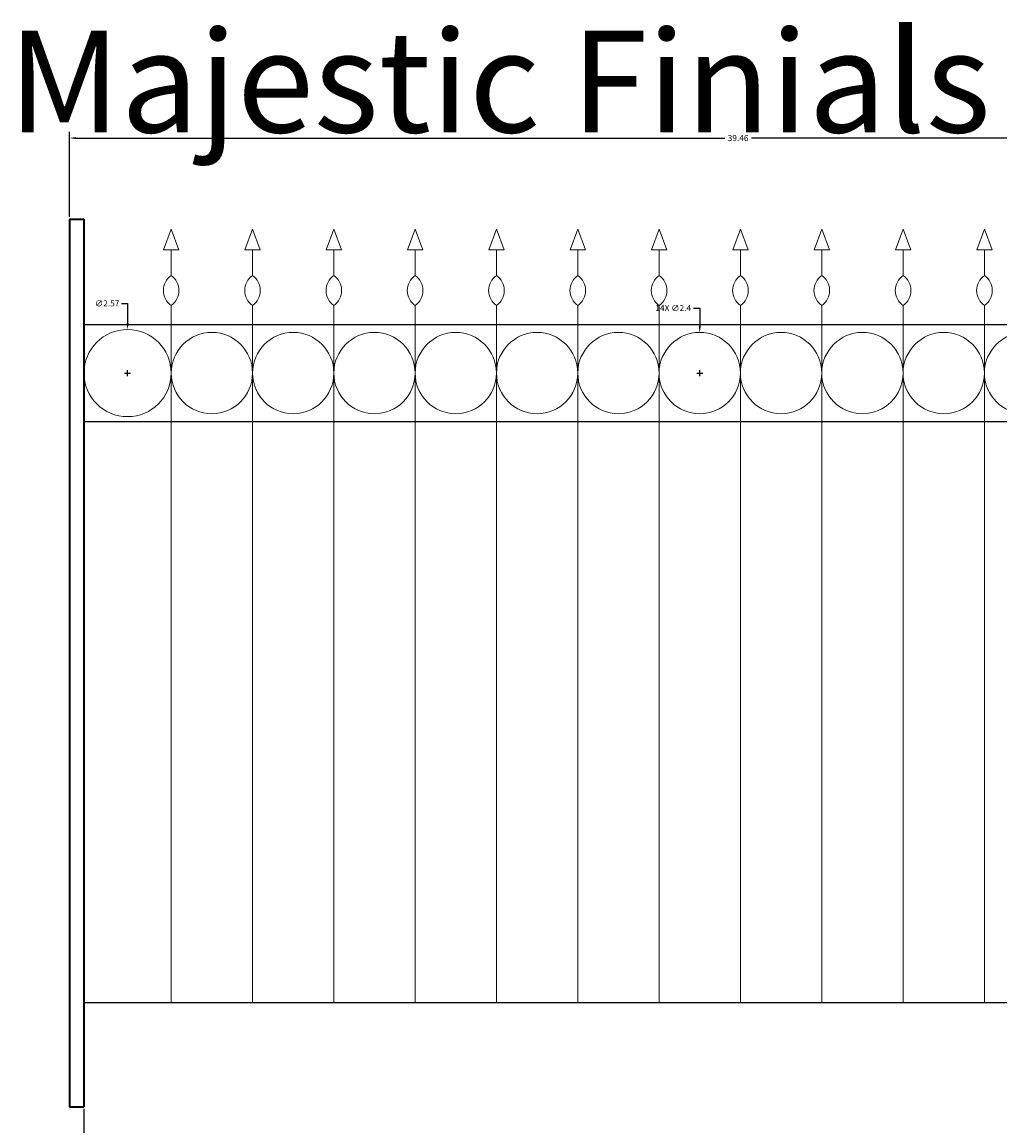
# Model space of a CAD drawing. Units: inches. Extents: x 756 to 915, y 488 to 695.
# Tile 5 of 25: x 815 to 844, y 512 to 545. Entities that reach past the tile are written whole.
import ezdxf

# ---------------------------------------------------------------- set-up
doc = ezdxf.new("R2010")
doc.units = ezdxf.units.IN
doc.header["$MEASUREMENT"] = 0
for name, color, linetype, lineweight in [('L-ANNO-TEXT', 7, 'Continuous', 25), ('L-FENC-PCKT', 7, 'Continuous', 18), ('L-FENC-POST', 7, 'Continuous', 35), ('L-FENC-RAIL', 7, 'Continuous', 25), ('L-FENC-RING', 7, 'Continuous', 18), ('M-DIMS', 2, 'Continuous', 18)]:
    doc.layers.add(name, color=color, linetype=linetype, lineweight=lineweight)
doc.styles.get("Standard").update_dxf_attribs({"font": 'arial.ttf'})
doc.dimstyles.get("Standard").update_dxf_attribs({"dimtxt": 0.18, "dimasz": 0.18, "dimexe": 0.18, "dimexo": 0.0625, "dimgap": 0.09, "dimtad": 0, "dimtih": 1, "dimtoh": 1, "dimdec": 0, "dimzin": 0, "dimdsep": 46, "dimlunit": 3, "dimtxsty": 'Standard', "dimcen": 0.09, "dimadec": 0, "dimazin": 0, "dimtfac": 1, "dimtdec": 0, "dimtofl": 0, "dimtmove": 0, "dimatfit": 3, "dimfxl": 1, "dimtolj": 1, "dimtzin": 0, "dimarcsym": 0})

# ---------------------------------------------------------------- blocks, each defined once
blk = doc.blocks.new('PICKET-MAJESTIC-FLUSH')
for p, q in [((0.231, 22.214), (0.231, 21.456)), ((0.231, 20.573), (0.231, 0))]:
    blk.add_line(p, q)
blk.add_lwpolyline([(0.231, 22.214), (0.004, 22.214), (0.231, 22.826), (0.458, 22.214)], close=True)
blk.add_lwpolyline([(0.231, 20.573, 0.522719), (0.231, 21.456, 0.522719)], format="xyb", close=True)
blk = doc.blocks.new('FENCE-POST-LEFT')
for p, q in [((0, 26.207), (0, 0)), ((0, 26.207), (0.426, 26.207)), ((0.426, 26.207), (0.426, 0)), ((0.426, 26.207), (0.426, 0)), ((0, 0), (0.426, 0))]:
    blk.add_line(p, q)
blk = doc.blocks.new('FENCE-PLUS-RING-BAND')
for centre, radius in [((1.286, 1.286), 1.286), ((3.773, 1.286), 1.2), ((6.173, 1.286), 1.2), ((8.572, 1.286), 1.2), ((10.972, 1.286), 1.2), ((13.372, 1.286), 1.2), ((15.772, 1.286), 1.2), ((18.172, 1.286), 1.2), ((20.572, 1.286), 1.2), ((22.972, 1.286), 1.2), ((25.372, 1.286), 1.2), ((27.772, 1.286), 1.2), ((30.172, 1.286), 1.2), ((32.572, 1.286), 1.2), ((34.971, 1.286), 1.2), ((37.388, 1.286), 1.217)]:
    blk.add_circle(centre, radius)
blk = doc.blocks.new('*D76')
at = {"layer": 'Defpoints', "color": 0, "transparency": 16777216}
for p in [(856.101, 541.142), (816.643, 538.752), (856.101, 538.752)]:
    blk.add_point(p, dxfattribs=at)
at = {"layer": 'M-DIMS', "color": 0, "lineweight": -2, "transparency": 16777216}
for p, q in [((816.643, 538.814), (816.643, 541.322)), ((856.101, 538.814), (856.101, 541.322)), ((816.823, 541.142), (835.978, 541.142)), ((855.921, 541.142), (836.765, 541.142))]:
    blk.add_line(p, q, dxfattribs=at)
at = {"layer": 'M-DIMS', "color": 0, "transparency": 16777216}
for points in [[(816.823, 541.172), (816.823, 541.112), (816.643, 541.142)], [(855.921, 541.172), (855.921, 541.112), (856.101, 541.142)]]:
    blk.add_solid(points, dxfattribs=at)
at = {"layer": 'M-DIMS', "color": 0, "transparency": 16777216, "insert": (836.372, 541.142), "char_height": 0.18, "attachment_point": 5}
blk.add_mtext('\\A1;39.46', dxfattribs=at)
blk = doc.blocks.new('*D78')
at = {"layer": 'Defpoints', "color": 0, "transparency": 16777216}
for p in [(817.069, 512.545), (855.674, 512.545), (855.674, 510.155)]:
    blk.add_point(p, dxfattribs=at)
at = {"layer": 'M-DIMS', "color": 0, "lineweight": -2, "transparency": 16777216}
for p, q in [((817.069, 512.482), (817.069, 509.975)), ((855.674, 512.482), (855.674, 509.975)), ((817.249, 510.155), (835.908, 510.155)), ((855.494, 510.155), (836.836, 510.155))]:
    blk.add_line(p, q, dxfattribs=at)
at = {"layer": 'M-DIMS', "color": 0, "transparency": 16777216}
for points in [[(817.249, 510.185), (817.249, 510.125), (817.069, 510.155)], [(855.494, 510.185), (855.494, 510.125), (855.674, 510.155)]]:
    blk.add_solid(points, dxfattribs=at)
at = {"layer": 'M-DIMS', "color": 0, "transparency": 16777216, "insert": (836.372, 510.155), "char_height": 0.18, "attachment_point": 5}
blk.add_mtext('\\A1;38.605', dxfattribs=at)
blk = doc.blocks.new('*D87')
at = {"layer": 'Defpoints', "color": 0, "transparency": 16777216}
for p in [(818.355, 535.491), (818.356, 532.918)]:
    blk.add_point(p, dxfattribs=at)
at = {"layer": 'M-DIMS', "color": 0, "lineweight": -2, "transparency": 16777216}
for p, q in [((818.175, 536.262), (818.355, 536.262)), ((818.355, 536.262), (818.355, 535.671)), ((818.266, 534.204), (818.446, 534.204)), ((818.356, 534.114), (818.356, 534.294))]:
    blk.add_line(p, q, dxfattribs=at)
at = {"layer": 'M-DIMS', "color": 0, "transparency": 16777216}
blk.add_solid([(818.385, 535.671), (818.325, 535.671), (818.355, 535.491)], dxfattribs=at)
at = {"layer": 'M-DIMS', "color": 0, "transparency": 16777216, "insert": (817.753, 536.262), "char_height": 0.18, "attachment_point": 5}
blk.add_mtext('\\A1;∅2.57', dxfattribs=at)
blk = doc.blocks.new('*D88')
at = {"layer": 'Defpoints', "color": 0, "transparency": 16777216}
for p in [(835.24, 535.404), (835.243, 533.004)]:
    blk.add_point(p, dxfattribs=at)
at = {"layer": 'M-DIMS', "color": 0, "lineweight": -2, "transparency": 16777216}
for p, q in [((835.059, 536.124), (835.239, 536.124)), ((835.239, 536.124), (835.24, 535.584)), ((835.151, 534.204), (835.331, 534.204)), ((835.241, 534.114), (835.241, 534.294))]:
    blk.add_line(p, q, dxfattribs=at)
at = {"layer": 'M-DIMS', "color": 0, "transparency": 16777216}
blk.add_solid([(835.27, 535.584), (835.21, 535.584), (835.24, 535.404)], dxfattribs=at)
at = {"layer": 'M-DIMS', "color": 0, "transparency": 16777216, "insert": (834.458, 536.124), "char_height": 0.18, "attachment_point": 5}
blk.add_mtext('\\A1;14X ∅2.4', dxfattribs=at)

msp = doc.modelspace()

# ---------------------------------------------------------------- linework, layer by layer
at = {"layer": 'L-FENC-RAIL'}
for p, q in [((817.0694, 535.6365), (855.6743, 535.6365)), ((817.0694, 532.7722), (855.6743, 532.7722)), ((817.0694, 515.6263), (855.6743, 515.6263))]:
    msp.add_line(p, q, dxfattribs=at)

# ---------------------------------------------------------------- block references
at = {"layer": 'L-FENC-PCKT'}
for p in [(819.411, 515.6267), (821.8109, 515.6267), (824.2108, 515.6267), (826.6107, 515.6267), (829.0106, 515.6267), (831.4106, 515.6267), (833.8105, 515.6267), (836.2104, 515.6267), (838.6103, 515.6267), (841.0102, 515.6267), (843.4101, 515.6267)]:
    msp.add_blockref('PICKET-MAJESTIC-FLUSH', p, dxfattribs=at)
at = {"layer": 'L-FENC-POST'}
msp.add_blockref('FENCE-POST-LEFT', (816.6431, 512.5446), dxfattribs=at)
at = {"layer": 'L-FENC-RING'}
msp.add_blockref('FENCE-PLUS-RING-BAND', (817.0693, 532.9183), dxfattribs=at)

# ---------------------------------------------------------------- texts
at = {"layer": 'L-ANNO-TEXT'}
msp.add_text('Majestic Finials', height=3, dxfattribs=at).set_placement((814.829, 541.3079))

# ---------------------------------------------------------------- dimensions: what is measured, and where the dimension line sits
at = {"layer": 'M-DIMS'}
for base, p1, p2, override, picture, middle in [((856.1009, 541.1415), (816.6428, 538.7515), (856.1009, 538.7515), {"dimdec": 2, "dimlfac": 1, "dimrnd": 0, "dimzin": 0, "dimdsep": 46, "dimlunit": 2}, '*D76', (836.3719, 541.1415)), ((855.6743, 510.1547), (817.0694, 512.5447), (855.6743, 512.5447), {"dimdec": 3, "dimlfac": 1, "dimrnd": 0, "dimzin": 0, "dimdsep": 46, "dimlunit": 2}, '*D78', (836.3719, 510.1547))]:
    dim = msp.add_linear_dim(base=base, p1=p1, p2=p2, dimstyle='Standard', override=override, dxfattribs=at)
    dim.commit()
    dim.dimension.update_dxf_attribs({"geometry": picture, "text_midpoint": middle})
dim = msp.add_diameter_dim_2p(p1=(818.3563, 532.9181), p2=(818.355, 535.4906), dimstyle='Standard', override={"dimdec": 2, "dimlfac": 1, "dimrnd": 0, "dimzin": 0, "dimdsep": 46, "dimlunit": 2}, dxfattribs=at)
dim.commit()
dim.dimension.update_dxf_attribs({"geometry": '*D87', "text_midpoint": (817.7529, 536.2623), "dimtype": 163})
dim = msp.add_diameter_dim_2p(p1=(835.2426, 533.0044), p2=(835.24, 535.4043), text='14X <>', dimstyle='Standard', override={"dimdec": 1, "dimlfac": 1, "dimrnd": 0, "dimzin": 0, "dimdsep": 46, "dimlunit": 2}, dxfattribs=at)
dim.commit()
dim.dimension.update_dxf_attribs({"geometry": '*D88', "text_midpoint": (834.4577, 536.1243), "dimtype": 163})

doc.saveas('drawing.dxf')
